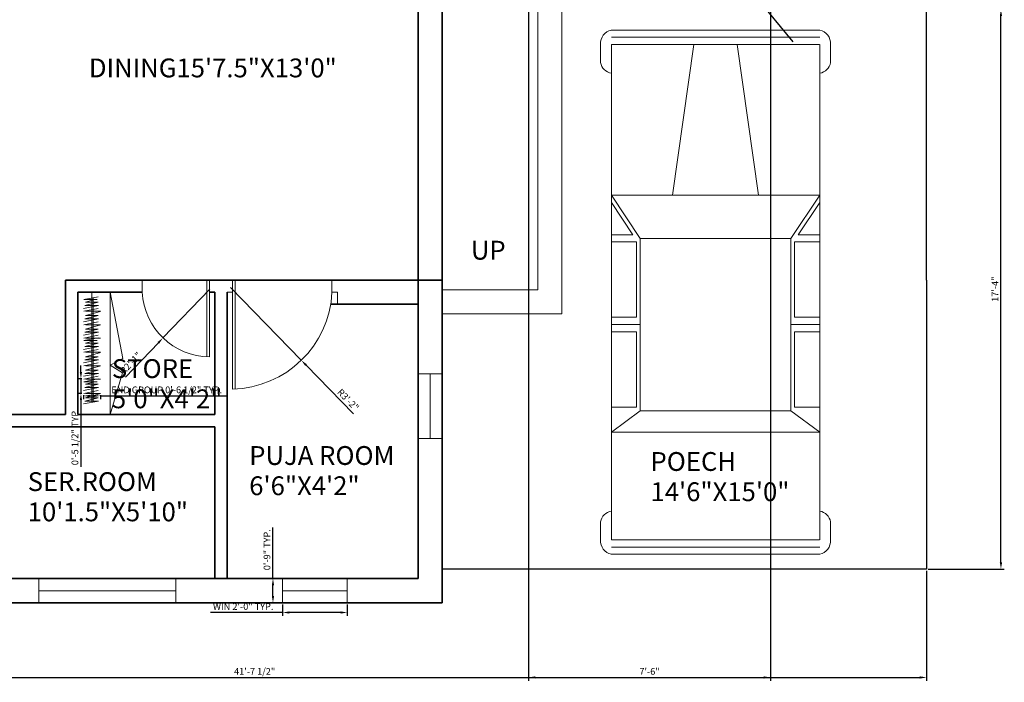
# Model space of a CAD drawing. Units: inches. Extents: x 1379 to 1989, y 1900 to 2397.
# Tile 2 of 3: x 1623 to 1989, y 1900 to 2146. Entities that reach past the tile are written whole.
import ezdxf

# ---------------------------------------------------------------- set-up
doc = ezdxf.new("R2010")
doc.units = ezdxf.units.IN
for name, color, linetype, lineweight in [('A-ANNO-DIMS', 2, 'Continuous', 18), ('A-ANNO-TEXT', 7, 'Continuous', 18), ('A-AREA-IDEN', 7, 'Continuous', 18), ('A-DOOR', 3, 'Continuous', 18), ('A-EQPM-VEHI', 8, 'Continuous', 13), ('A-FLOR', 7, 'Continuous', 25), ('A-FLOR-CASE', 9, 'Continuous', 18), ('A-FLOR-STRS', 7, 'Continuous', 18), ('A-GLAZ', 4, 'Continuous', 18), ('A-WALL', 7, 'Continuous', 35)]:
    doc.layers.add(name, color=color, linetype=linetype, lineweight=lineweight)
doc.styles.get("Standard").update_dxf_attribs({"font": 'arial.ttf'})
doc.dimstyles.new('ISO-25', dxfattribs={"dimtxt": 2.5, "dimasz": 2.5, "dimexe": 1.25, "dimexo": 0.625, "dimtad": 1, "dimlunit": 3, "dimtxsty": 'Standard', "dimcen": 2.5, "dimadec": 0, "dimazin": 0, "dimtfac": 1, "dimtmove": 0, "dimatfit": 3, "dimfxl": 1, "dimarcsym": 0})

# ---------------------------------------------------------------- blocks, each defined once
blk = doc.blocks.new('*U5')
for p, q in [((138.2, 1074.7), (307.8, 1074.7)), ((4818.1, 1074.7), (4648.5, 1074.7)), ((2.6, -10.3), (2.6, 974.1)), ((70.4, -10.5), (70.4, 973)), ((138.2, -10.3), (138.2, 971.4)), ((138.3, 973), (409.5, 973)), ((409.5, 973), (4580.7, 973)), ((1562.5, -10.5), (1562.5, 973)), ((1562.5, 973), (1969.5, 701.7)), ((1630.4, 973), (1935.6, 769.5)), ((1935.6, 769.5), (1935.6, 973)), ((2003.4, 973), (2003.4, 735.6)), ((2715.6, 735.6), (2715.6, 973)), ((2783.4, 701.7), (2783.4, 973)), ((2851.2, 973), (2851.2, 735.6)), ((3563.3, 735.6), (3563.3, 973)), ((3597.3, 701.7), (3800.7, 973)), ((3800.7, -10.5), (3800.7, 973)), ((4818, 973), (4546.8, 973)), ((4818.1, -10.3), (4818.1, 971.4)), ((4885.9, -10.5), (4885.9, 973)), ((4953.7, -10.3), (4953.7, 974.1)), ((1969.5, 701.7), (3597.3, 701.7)), ((1969.5, -10.5), (1969.5, 701.7)), ((2003.4, 735.6), (2715.6, 735.6)), ((2851.2, 735.6), (3563.3, 735.6)), ((3597.3, -10.5), (3597.3, 701.7)), ((138.2, 193), (1562.5, 396.4)), ((2.6, -10.7), (2.6, -995.1)), ((70.4, -10.5), (70.4, -993.9)), ((138.2, -10.7), (138.2, -992.4)), ((1562.5, -10.5), (1562.5, -993.9)), ((1969.5, -10.5), (1969.5, -722.6)), ((3597.3, -10.5), (3597.3, -722.6)), ((3800.7, -10.5), (3800.7, -993.9)), ((4818.1, -10.7), (4818.1, -992.4)), ((4885.9, -10.5), (4885.9, -993.9)), ((4953.7, -10.7), (4953.7, -995.1)), ((138.2, -214), (1562.5, -417.4)), ((1562.5, -993.9), (1969.5, -722.6)), ((1969.5, -722.6), (3597.3, -722.6)), ((2783.4, -722.6), (2783.4, -993.9)), ((3597.3, -722.6), (3800.7, -993.9)), ((1630.4, -993.9), (1935.6, -790.5)), ((1935.6, -790.5), (1935.6, -993.9)), ((2003.4, -993.9), (2003.4, -756.6)), ((2003.4, -756.6), (2715.6, -756.6)), ((2715.6, -756.6), (2715.6, -993.9)), ((2851.2, -756.6), (3563.3, -756.6)), ((2851.2, -993.9), (2851.2, -756.6)), ((3563.3, -756.6), (3563.3, -993.9)), ((138.3, -993.9), (409.5, -993.9)), ((409.5, -993.9), (4580.7, -993.9)), ((4818, -993.9), (4546.8, -993.9)), ((138.2, -1095.7), (307.8, -1095.7)), ((4818.1, -1095.7), (4648.5, -1095.7))]:
    blk.add_line(p, q)
for centre, radius, start, end in [((128.5, 946.4), 128.6, 85.64554, 168.0943), ((290.8, 956), 119.9, 8.13011, 81.86996), ((4665.5, 956), 119.9, 98.13004, 171.8699), ((4827.9, 946.4), 128.6, 11.90574, 94.35446), ((128.5, -967.4), 128.6, 191.9057, 274.3545), ((290.8, -977), 119.9, 278.13, 351.8699), ((4665.5, -977), 119.9, 188.1301, 261.87), ((4827.9, -967.4), 128.6, 265.6455, 348.0943)]:
    blk.add_arc(centre, radius, start, end)
blk = doc.blocks.new('WIN-51IN')
for p, q in [((0, 51), (9, 51)), ((4.5, 51), (4.5, 0)), ((9, 0), (0, 0)), ((4.5, 0), (9, 0))]:
    blk.add_line(p, q)
blk = doc.blocks.new('WIN-24IN')
for p, q in [((0, 24), (9, 24)), ((4.5, 24), (4.5, 0)), ((9, 0), (0, 0)), ((4.5, 0), (9, 0))]:
    blk.add_line(p, q)
blk = doc.blocks.new('CLOSET-GARMENT-CLUSTER')
for p, q in [((0, 6.34), (1.58, 0.7)), ((1.58, 0.7), (1.58, 5.41)), ((1.58, 5.41), (2.79, 0.56)), ((2.79, 0.56), (2.79, 5.59)), ((2.79, 5.59), (3.87, 0)), ((3.87, 5.45), (4.94, 0.19)), ((4.94, 0.83), (4.94, 6.28))]:
    blk.add_line(p, q)
blk = doc.blocks.new('CLOSET-GARMENT-CLUSTER-END')
for p, q in [((0, 5.45), (1.07, 0.19)), ((1.07, 0.19), (1.07, 5.08)), ((1.07, 0.83), (1.07, 4.19)), ((1.07, 4.19), (2.05, 0.7)), ((2.05, 0.7), (2.05, 5.41)), ((2.05, 5.41), (3.26, 0.56)), ((3.26, 0.56), (3.26, 5.59)), ((3.26, 5.59), (4.34, 0)), ((4.34, 5.45), (5.41, 0.19)), ((5.41, 0.83), (5.41, 6.28))]:
    blk.add_line(p, q)
blk = doc.blocks.new('*D17')
at = {"layer": 'A-ANNO-DIMS', "color": 0, "lineweight": -2, "transparency": 16777216}
for p, q in [((1720.58, 1928.96), (1720.58, 1924.73)), ((1744.58, 1928.96), (1744.58, 1924.73)), ((1720.58, 1925.98), (1693.73, 1925.98)), ((1742.08, 1925.98), (1723.08, 1925.98))]:
    blk.add_line(p, q, dxfattribs=at)
at = {"layer": 'A-ANNO-DIMS', "color": 0, "transparency": 16777216}
for points in [[(1723.08, 1926.4), (1723.08, 1925.56), (1720.58, 1925.98)], [(1742.08, 1926.4), (1742.08, 1925.56), (1744.58, 1925.98)]]:
    blk.add_solid(points, dxfattribs=at)
at = {"layer": 'Defpoints', "color": 0, "transparency": 16777216}
for p in [(1720.58, 1929.58), (1744.58, 1929.58), (1720.58, 1925.98)]:
    blk.add_point(p, dxfattribs=at)
at = {"layer": 'A-ANNO-DIMS', "color": 0, "transparency": 16777216, "insert": (1705.9, 1927.88), "char_height": 2.5, "attachment_point": 5}
blk.add_mtext('WIN 2\'-0" TYP.', dxfattribs=at)
blk = doc.blocks.new('*D18')
at = {"layer": 'A-ANNO-DIMS', "color": 0, "lineweight": -2, "transparency": 16777216}
for p, q in [((1716.98, 1938.58), (1716.98, 1957.57)), ((1719.95, 1938.58), (1715.73, 1938.58)), ((1716.98, 1932.08), (1716.98, 1936.08)), ((1719.95, 1929.58), (1715.73, 1929.58))]:
    blk.add_line(p, q, dxfattribs=at)
at = {"layer": 'A-ANNO-DIMS', "color": 0, "transparency": 16777216}
for points in [[(1716.56, 1936.08), (1717.39, 1936.08), (1716.98, 1938.58)], [(1716.56, 1932.08), (1717.39, 1932.08), (1716.98, 1929.58)]]:
    blk.add_solid(points, dxfattribs=at)
at = {"layer": 'Defpoints', "color": 0, "transparency": 16777216}
for p in [(1716.98, 1938.58), (1720.58, 1938.58), (1720.58, 1929.58)]:
    blk.add_point(p, dxfattribs=at)
at = {"layer": 'A-ANNO-DIMS', "color": 0, "transparency": 16777216, "insert": (1715.08, 1949.33), "char_height": 2.5, "attachment_point": 5, "rotation": 90}
blk.add_mtext('0\'-9" TYP.', dxfattribs=at)
blk = doc.blocks.new('*D27')
at = {"layer": 'A-ANNO-DIMS', "color": 0, "lineweight": -2, "transparency": 16777216}
for p, q in [((1646.54, 2006.85), (1646.54, 2005.28)), ((1649.04, 2006.53), (1650.32, 2006.53)), ((1652.82, 2006.85), (1652.82, 2005.28)), ((1652.82, 2006.53), (1699.63, 2006.53))]:
    blk.add_line(p, q, dxfattribs=at)
at = {"layer": 'A-ANNO-DIMS', "color": 0, "transparency": 16777216}
for points in [[(1649.04, 2006.95), (1649.04, 2006.11), (1646.54, 2006.53)], [(1650.32, 2006.95), (1650.32, 2006.11), (1652.82, 2006.53)]]:
    blk.add_solid(points, dxfattribs=at)
at = {"layer": 'Defpoints', "color": 0, "transparency": 16777216}
for p in [(1646.54, 2007.47), (1652.82, 2007.47), (1652.82, 2006.53)]:
    blk.add_point(p, dxfattribs=at)
at = {"layer": 'A-ANNO-DIMS', "color": 0, "transparency": 16777216, "insert": (1677.48, 2008.45), "char_height": 2.5, "attachment_point": 5}
blk.add_mtext('END GROUP 0\'-6 1/2" TYP.', dxfattribs=at)
blk = doc.blocks.new('*D28')
at = {"layer": 'A-ANNO-DIMS', "color": 0, "lineweight": -2, "transparency": 16777216}
for p, q in [((1645.6, 2015.38), (1645.6, 2017.88)), ((1645.92, 2012.88), (1644.35, 2012.88)), ((1645.6, 2012.88), (1645.6, 2007.47)), ((1645.92, 2007.47), (1644.35, 2007.47)), ((1645.6, 2004.97), (1645.6, 1980.16))]:
    blk.add_line(p, q, dxfattribs=at)
at = {"layer": 'A-ANNO-DIMS', "color": 0, "transparency": 16777216}
for points in [[(1645.18, 2015.38), (1646.01, 2015.38), (1645.6, 2012.88)], [(1645.18, 2004.97), (1646.01, 2004.97), (1645.6, 2007.47)]]:
    blk.add_solid(points, dxfattribs=at)
at = {"layer": 'Defpoints', "color": 0, "transparency": 16777216}
for p in [(1646.54, 2012.88), (1645.6, 2007.47), (1646.54, 2007.47)]:
    blk.add_point(p, dxfattribs=at)
at = {"layer": 'A-ANNO-DIMS', "color": 0, "transparency": 16777216, "insert": (1643.68, 1991.32), "char_height": 2.5, "attachment_point": 5, "rotation": 90}
blk.add_mtext('0\'-5 1/2" TYP.', dxfattribs=at)
blk = doc.blocks.new('*D29')
at = {"layer": 'A-ANNO-DIMS', "color": 0, "lineweight": -2, "transparency": 16777216}
for p, q in [((1959.91, 1941.48), (1959.91, 1900.58)), ((1460.41, 1928.96), (1460.41, 1900.58)), ((1462.91, 1901.83), (1957.41, 1901.83))]:
    blk.add_line(p, q, dxfattribs=at)
at = {"layer": 'A-ANNO-DIMS', "color": 0, "transparency": 16777216}
for points in [[(1462.91, 1902.24), (1462.91, 1901.41), (1460.41, 1901.83)], [(1957.41, 1902.24), (1957.41, 1901.41), (1959.91, 1901.83)]]:
    blk.add_solid(points, dxfattribs=at)
at = {"layer": 'Defpoints', "color": 0, "transparency": 16777216}
for p in [(1959.91, 1942.11), (1460.41, 1929.58), (1959.91, 1901.83)]:
    blk.add_point(p, dxfattribs=at)
at = {"layer": 'A-ANNO-DIMS', "color": 0, "transparency": 16777216, "insert": (1710.16, 1903.75), "char_height": 2.5, "attachment_point": 5}
blk.add_mtext('41\'-7 1/2"', dxfattribs=at)
blk = doc.blocks.new('*D32')
at = {"layer": 'A-ANNO-DIMS', "color": 0, "lineweight": -2, "transparency": 16777216}
for p, q in [((1960.54, 2150.31), (1988.81, 2150.31)), ((1987.56, 1944.61), (1987.56, 2147.81)), ((1960.54, 1942.11), (1988.81, 1942.11))]:
    blk.add_line(p, q, dxfattribs=at)
at = {"layer": 'A-ANNO-DIMS', "color": 0, "transparency": 16777216}
for points in [[(1987.14, 2147.81), (1987.98, 2147.81), (1987.56, 2150.31)], [(1987.14, 1944.61), (1987.98, 1944.61), (1987.56, 1942.11)]]:
    blk.add_solid(points, dxfattribs=at)
at = {"layer": 'Defpoints', "color": 0, "transparency": 16777216}
for p in [(1959.91, 2150.31), (1987.56, 2150.31), (1959.91, 1942.11)]:
    blk.add_point(p, dxfattribs=at)
at = {"layer": 'A-ANNO-DIMS', "color": 0, "transparency": 16777216, "insert": (1985.68, 2046.21), "char_height": 2.5, "attachment_point": 5, "rotation": 90}
blk.add_mtext('17\'-4"', dxfattribs=at)
blk = doc.blocks.new('*D42')
at = {"layer": 'A-ANNO-DIMS', "color": 0, "lineweight": -2, "transparency": 16777216}
for p, q in [((1811.97, 2310.14), (1811.97, 1900.58)), ((1901.92, 2222.46), (1901.92, 1900.58)), ((1814.47, 1901.83), (1899.42, 1901.83))]:
    blk.add_line(p, q, dxfattribs=at)
at = {"layer": 'A-ANNO-DIMS', "color": 0, "transparency": 16777216}
for points in [[(1814.47, 1902.24), (1814.47, 1901.41), (1811.97, 1901.83)], [(1899.42, 1902.24), (1899.42, 1901.41), (1901.92, 1901.83)]]:
    blk.add_solid(points, dxfattribs=at)
at = {"layer": 'Defpoints', "color": 0, "transparency": 16777216}
for p in [(1811.97, 2310.77), (1901.92, 2223.09), (1901.92, 1901.83)]:
    blk.add_point(p, dxfattribs=at)
at = {"layer": 'A-ANNO-DIMS', "color": 0, "transparency": 16777216, "insert": (1856.94, 1903.73), "char_height": 2.5, "attachment_point": 5}
blk.add_mtext('7\'-6"', dxfattribs=at)
blk = doc.blocks.new('*D44')
at = {"layer": 'A-ANNO-DIMS', "color": 0, "lineweight": -2, "transparency": 16777216}
for p, q in [((1853.31, 2207.74), (1875.14, 2181.12)), ((1910.32, 2138.22), (1876.73, 2179.19))]:
    blk.add_line(p, q, dxfattribs=at)
at = {"layer": 'A-ANNO-DIMS', "color": 0, "transparency": 16777216}
blk.add_solid([(1875.47, 2181.38), (1874.82, 2180.85), (1876.73, 2179.19)], dxfattribs=at)
at = {"layer": 'Defpoints', "color": 0, "transparency": 16777216}
for p in [(1876.73, 2179.19), (1910.32, 2138.22)]:
    blk.add_point(p, dxfattribs=at)
at = {"layer": 'A-ANNO-DIMS', "color": 0, "transparency": 16777216, "insert": (1858.04, 2204.97), "char_height": 2.5, "attachment_point": 5, "rotation": 309.3523}
blk.add_mtext('R4\'-5"', dxfattribs=at)
blk = doc.blocks.new('*D45')
at = {"layer": 'A-ANNO-DIMS', "color": 0, "lineweight": -2, "transparency": 16777216}
for p, q in [((1701.16, 2046.86), (1727.51, 2019.78)), ((1746.91, 1999.84), (1729.26, 2017.99))]:
    blk.add_line(p, q, dxfattribs=at)
at = {"layer": 'A-ANNO-DIMS', "color": 0, "transparency": 16777216}
blk.add_solid([(1729.56, 2018.28), (1728.96, 2017.7), (1727.51, 2019.78)], dxfattribs=at)
at = {"layer": 'Defpoints', "color": 0, "transparency": 16777216}
for p in [(1701.16, 2046.86), (1727.51, 2019.78)]:
    blk.add_point(p, dxfattribs=at)
at = {"layer": 'A-ANNO-DIMS', "color": 0, "transparency": 16777216, "insert": (1744.69, 2004.85), "char_height": 2.5, "attachment_point": 5, "rotation": 314.2148}
blk.add_mtext('R3\'-2"', dxfattribs=at)
blk = doc.blocks.new('*D50')
at = {"layer": 'A-ANNO-DIMS', "color": 0, "lineweight": -2, "transparency": 16777216}
for p, q in [((1693.49, 2046.19), (1676.1, 2028.08)), ((1662.11, 2013.5), (1674.37, 2026.27))]:
    blk.add_line(p, q, dxfattribs=at)
at = {"layer": 'A-ANNO-DIMS', "color": 0, "transparency": 16777216}
blk.add_solid([(1674.07, 2026.56), (1674.67, 2025.98), (1676.1, 2028.08)], dxfattribs=at)
at = {"layer": 'Defpoints', "color": 0, "transparency": 16777216}
for p in [(1693.49, 2046.19), (1676.1, 2028.08)]:
    blk.add_point(p, dxfattribs=at)
at = {"layer": 'A-ANNO-DIMS', "color": 0, "transparency": 16777216, "insert": (1664.32, 2018.51), "char_height": 2.5, "attachment_point": 5, "rotation": 46.1693}
blk.add_mtext('R2\'-1"', dxfattribs=at)

msp = doc.modelspace()

# ---------------------------------------------------------------- linework, layer by layer
at = {"layer": 'A-DOOR'}
for p, q in [((1668.61, 2049.535), (1668.41, 2049.535)), ((1668.41, 2049.535), (1668.41, 2045.082)), ((1692.41, 2021.082), (1692.41, 2049.535)), ((1693.41, 2049.535), (1693.41, 2045.082)), ((1701.91, 2049.582), (1701.91, 2045.082)), ((1702.91, 2009.115), (1702.91, 2049.582)), ((1702.91, 2049.582), (1738.91, 2049.582)), ((1738.91, 2049.582), (1738.91, 2045.082)), ((1738.91, 2049.582), (1738.91, 2045.082)), ((1693.41, 2045.082), (1693.41, 2021.082)), ((1693.41, 2040.582), (1693.41, 2045.082)), ((1701.91, 2045.082), (1699.91, 2045.082)), ((1701.91, 2045.082), (1701.91, 2009.082)), ((1738.91, 2045.082), (1740.91, 2045.082)), ((1740.91, 2045.082), (1740.91, 2040.582))]:
    msp.add_line(p, q, dxfattribs=at)
for centre, radius, start, end in [((1693.491, 2046.187), 25.105, 182.52281, 269.81547), ((1701.162, 2046.865), 37.791, 271.13498, 357.29537)]:
    msp.add_arc(centre, radius, start, end, dxfattribs=at)
at = {"layer": 'A-FLOR'}
for p, q in [((1959.91, 2049.582), (1959.91, 2150.308)), ((1959.91, 2049.582), (1959.91, 1976.308)), ((1959.91, 1976.308), (1959.91, 1942.11)), ((1959.91, 1942.11), (1779.91, 1942.11))]:
    msp.add_line(p, q, dxfattribs=at)
at = {"layer": 'A-FLOR-CASE'}
for p, q in [((1649.61, 2045.082), (1649.61, 2004.145)), ((1650.098, 2043.027), (1650.098, 2028.024)), ((1656.41, 2045.082), (1656.41, 1999.582)), ((1656.41, 2045.082), (1661.148, 2020.487)), ((1650.098, 2027.762), (1650.098, 2012.759)), ((1661.148, 2020.487), (1656.41, 2017.924)), ((1656.41, 2017.924), (1661.02, 2015.106)), ((1661.02, 2015.106), (1656.41, 1999.582)), ((1650.098, 2012.497), (1650.098, 2004.239)), ((1651.947, 2005.842), (1647.1, 2004.629)), ((1652.879, 2007.424), (1647.24, 2005.842)), ((1647.24, 2005.842), (1651.947, 2005.842)), ((1652.133, 2004.629), (1646.541, 2003.557)), ((1647.1, 2004.629), (1652.133, 2004.629))]:
    msp.add_line(p, q, dxfattribs=at)
at = {"layer": 'A-FLOR-STRS'}
for p, q in [((1815.368, 2046.02), (1815.368, 2150.308)), ((1824.368, 2150.308), (1824.368, 2045.838)), ((1779.91, 2046.02), (1815.368, 2046.02)), ((1824.368, 2045.838), (1824.368, 2038.106)), ((1779.91, 2037.02), (1824.368, 2037.02)), ((1824.368, 2037.02), (1824.368, 2038.106))]:
    msp.add_line(p, q, dxfattribs=at)
at = {"layer": 'A-WALL'}
for p, q in [((1770.91, 2040.582), (1770.91, 2312.038)), ((1779.91, 2049.582), (1779.91, 2150.308)), ((1699.91, 2049.582), (1639.91, 2049.582)), ((1639.91, 2049.582), (1639.91, 1999.582)), ((1699.91, 2049.582), (1701.91, 2049.582)), ((1701.91, 2049.582), (1779.91, 2049.582)), ((1779.91, 2049.582), (1779.91, 1938.582)), ((1644.41, 2045.082), (1644.41, 1999.582)), ((1668.41, 2045.082), (1644.41, 2045.082)), ((1695.41, 2045.082), (1693.41, 2045.082)), ((1695.41, 1999.582), (1695.41, 2045.082)), ((1699.91, 1999.582), (1699.91, 2045.082)), ((1738.426, 2040.582), (1770.91, 2040.582)), ((1770.91, 2040.582), (1770.91, 1938.582)), ((1578.41, 1999.582), (1639.91, 1999.582)), ((1644.41, 1999.582), (1695.41, 1999.582)), ((1699.91, 1999.582), (1699.91, 1938.582)), ((1578.41, 1995.082), (1695.41, 1995.082)), ((1695.41, 1995.082), (1695.41, 1938.582)), ((1618.41, 1938.582), (1770.91, 1938.582)), ((1779.851, 1929.582), (1779.91, 1938.582)), ((1565.41, 1929.582), (1744.577, 1929.582)), ((1744.577, 1929.582), (1779.851, 1929.582))]:
    msp.add_line(p, q, dxfattribs=at)

# ---------------------------------------------------------------- block references
at = {"layer": 'A-EQPM-VEHI', "xscale": 0.0393700787401575, "yscale": 0.0393700787401575, "zscale": 0.0393700787401575, "rotation": 270}
msp.add_blockref('*U5', (1881.891, 2142.661), dxfattribs=at)
at = {"layer": 'A-FLOR-CASE'}
for name, p, rotation in [('CLOSET-GARMENT-CLUSTER-END', (1646.541, 2043.412), 269.9999999999919), ('CLOSET-GARMENT-CLUSTER', (1646.541, 2037.953), 269.9999999999865), ('CLOSET-GARMENT-CLUSTER', (1646.541, 2032.964), 269.9999999999954), ('CLOSET-GARMENT-CLUSTER-END', (1646.541, 2028.148), 270.0000000000029), ('CLOSET-GARMENT-CLUSTER', (1646.541, 2022.689), 269.999999999993), ('CLOSET-GARMENT-CLUSTER', (1646.541, 2017.699), 270.0000000000065), ('CLOSET-GARMENT-CLUSTER-END', (1646.541, 2012.883), 270.0000000000021)]:
    msp.add_blockref(name, p, dxfattribs=dict(at, rotation=rotation))
at = {"layer": 'A-GLAZ', "extrusion": (0, 0, -1), "zscale": -1}
msp.add_blockref('WIN-24IN', (-1779.91, 1990.747), dxfattribs=at)
at = {"layer": 'A-GLAZ'}
for name, p, rotation in [('WIN-51IN', (1680.913, 1929.581), 89.99999999999909), ('WIN-24IN', (1744.577, 1929.581), 89.99999999999793)]:
    msp.add_blockref(name, p, dxfattribs=dict(at, rotation=rotation))

# ---------------------------------------------------------------- texts
at = {"layer": 'A-ANNO-TEXT'}
msp.add_text('UP', height=7, dxfattribs=at).set_placement((1790.541, 2057.211))
at = {"layer": 'A-AREA-IDEN'}
for s, p in [('DINING15\'7.5"X13\'0"', (1648.549, 2124.992)), ('STORE', (1657.11, 2013.184)), ('5\'0"X4\'2"', (1657.11, 2001.939)), ('PUJA ROOM', (1708.147, 1980.859)), ('POECH', (1857.304, 1978.634)), ('SER.ROOM', (1625.799, 1971.147)), ('6\'6"X4\'2"', (1708.147, 1969.614)), ('14\'6"X15\'0"', (1857.304, 1967.389)), ('10\'1.5"X5\'10"', (1625.799, 1959.902))]:
    msp.add_text(s, height=7, dxfattribs=at).set_placement(p)

# ---------------------------------------------------------------- dimensions: what is measured, and where the dimension line sits
at = {"layer": 'A-ANNO-DIMS'}
for base, p1, p2, picture, middle in [((1901.918, 1901.828), (1811.97, 2310.77), (1901.918, 2223.089), '*D42', (1856.944, 1903.729)), ((1959.91, 1901.828), (1460.41, 1929.582), (1959.91, 1942.11), '*D29', (1710.16, 1903.745))]:
    dim = msp.add_linear_dim(base=base, p1=p1, p2=p2, dimstyle='ISO-25', override={"dimdec": 1, "dimlfac": 1, "dimrnd": 0, "dimzin": 1, "dimdsep": 46, "dimlunit": 4, "dimfrac": 2}, dxfattribs=at)
    dim.commit()
    dim.dimension.update_dxf_attribs({"geometry": picture, "text_midpoint": middle})
for center, mpoint, picture, middle in [((1910.322, 2138.221), (1876.73, 2179.185), '*D44', (1856.575, 2203.764)), ((1693.491, 2046.187), (1676.105, 2028.076), '*D50', (1665.673, 2017.21)), ((1701.162, 2046.865), (1727.515, 2019.779), '*D45', (1743.327, 2003.528))]:
    dim = msp.add_radius_dim(center=center, mpoint=mpoint, dimstyle='ISO-25', override={"dimdec": 1, "dimlfac": 1, "dimrnd": 0, "dimzin": 1, "dimdsep": 46, "dimlunit": 4, "dimfrac": 2}, dxfattribs=at)
    dim.commit()
    dim.dimension.update_dxf_attribs({"geometry": picture, "text_midpoint": middle, "dimtype": 164})
dim = msp.add_linear_dim(base=(1987.56, 2150.308), p1=(1959.91, 1942.11), p2=(1959.91, 2150.308), angle=90, dimstyle='ISO-25', override={"dimdec": 1, "dimlfac": 1, "dimrnd": 0, "dimzin": 1, "dimdsep": 46, "dimlunit": 4, "dimfrac": 2}, dxfattribs=at)
dim.commit()
dim.dimension.update_dxf_attribs({"geometry": '*D32', "text_midpoint": (1985.68, 2046.209)})
for base, p1, p2, angle, text, picture, middle in [((1645.598, 2007.474), (1646.541, 2012.883), (1646.541, 2007.474), 270, '<> TYP.', '*D28', (1643.681, 1991.317)), ((1652.824, 2006.531), (1646.541, 2007.474), (1652.824, 2007.474), 0, 'END GROUP <> TYP.', '*D27', (1677.476, 2008.45)), ((1716.977, 1938.582), (1720.577, 1929.582), (1720.577, 1938.582), 90, '<> TYP.', '*D18', (1715.075, 1949.326)), ((1720.577, 1925.982), (1744.577, 1929.582), (1720.577, 1929.582), 180, 'WIN <> TYP.', '*D17', (1705.902, 1927.883))]:
    dim = msp.add_linear_dim(base=base, p1=p1, p2=p2, angle=angle, text=text, dimstyle='ISO-25', override={"dimdec": 1, "dimlfac": 1, "dimrnd": 0, "dimzin": 1, "dimdsep": 46, "dimlunit": 4, "dimfrac": 2}, dxfattribs=at)
    dim.commit()
    dim.dimension.update_dxf_attribs({"geometry": picture, "text_midpoint": middle})

doc.saveas('drawing.dxf')
